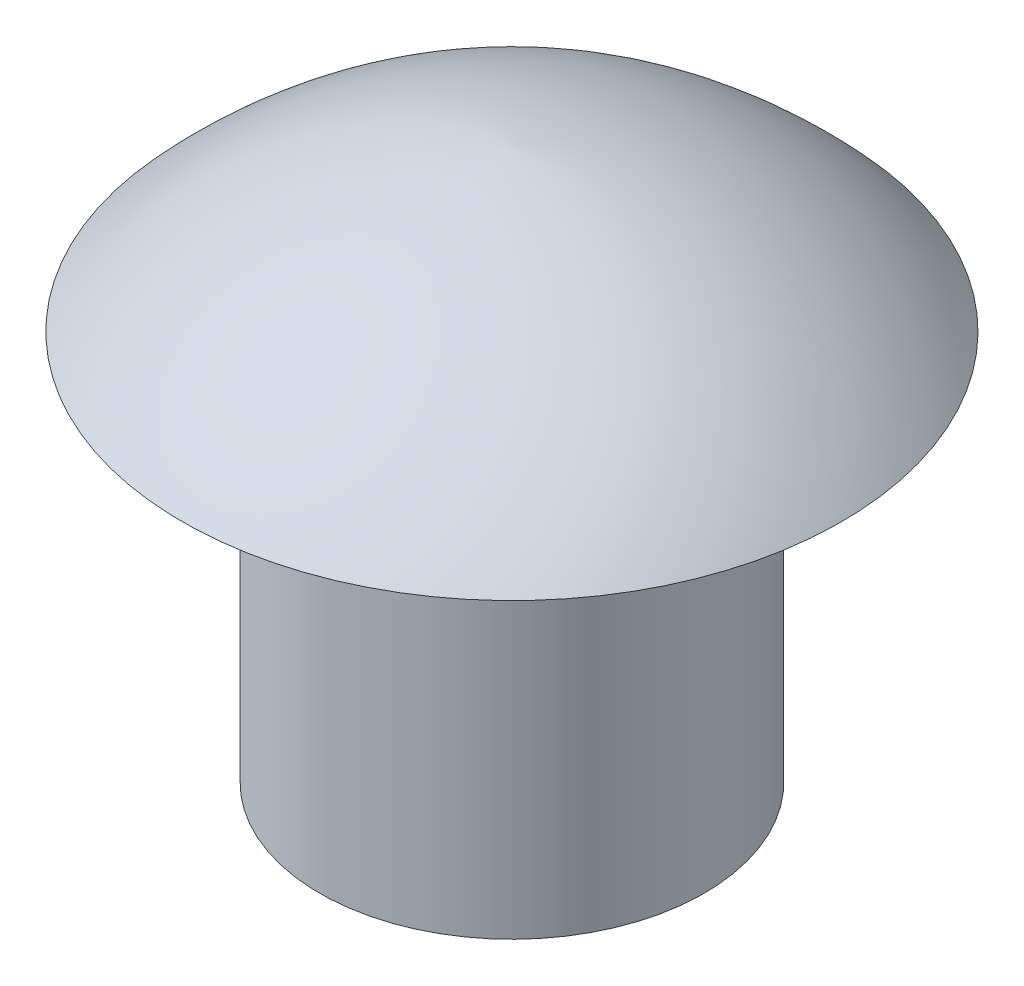
from build123d import *


with BuildPart() as part:
    # End Cap Half Profile → End Cap Revolve (revolve)
    with BuildSketch(Plane.XY, mode=Mode.PRIVATE) as end_cap_revolve_sk:
        with BuildLine():
            Line((0, 0), (1.75, 0))
            Line((1.75, 0), (1.75, 3.553882595))
            Line((1.75, 3.553882595), (3, 3.553882595))
            ThreePointArc((3, 3.553882595), (1.638702903, 4.564683294), (0, 5))
            Line((0, 5), (0, 0))
        make_face()
    revolve(end_cap_revolve_sk.sketch.rotate(Axis((0, 0, 0), (0, 1, 0)), 90), axis=Axis((0, 0, 0), (0, 1, 0)))


solid = part.part
